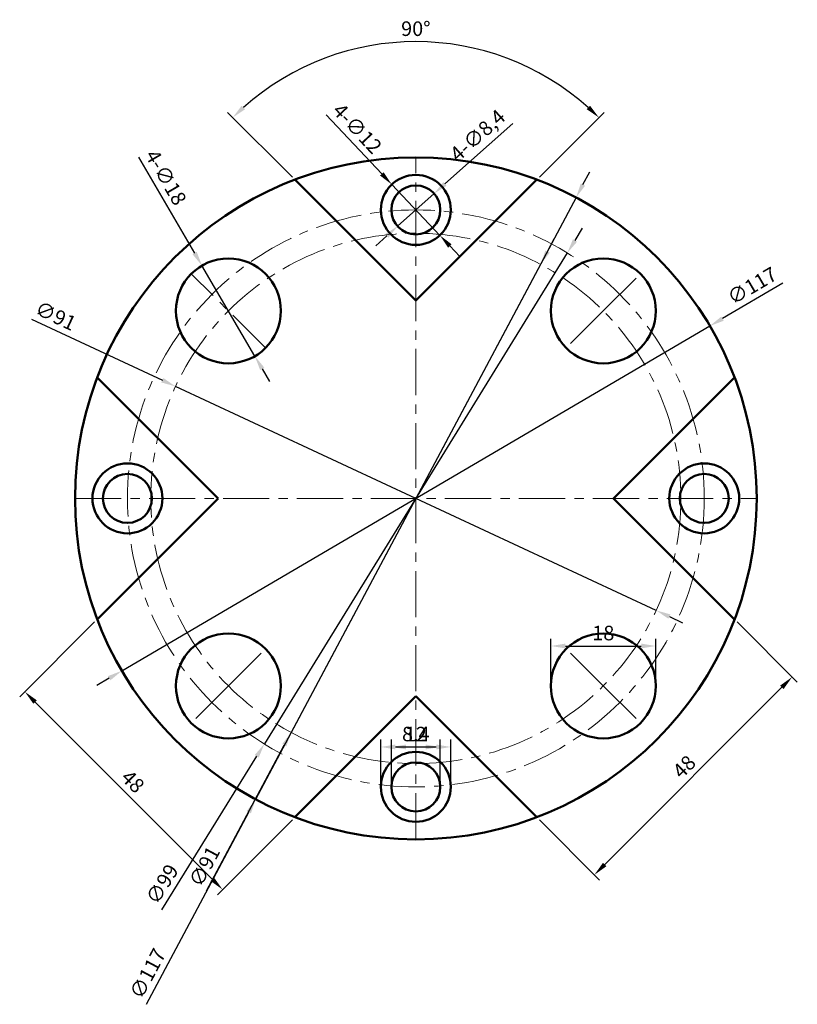
# Model space of a CAD drawing. Units: millimetres. Extents: x 3034 to 3167, y 1610 to 1779.
import ezdxf

# ---------------------------------------------------------------- set-up
doc = ezdxf.new("R2010")
doc.units = ezdxf.units.MM
doc.linetypes.add('CENTER', pattern=[50.8, 31.75, -6.35, 6.35, -6.35])
for name, color, linetype, lineweight in [('M-CNTR', 4, 'CENTER', 18), ('M-DIMS', 2, 'Continuous', 25), ('M-OUTL', 7, 'Continuous', 50)]:
    doc.layers.add(name, color=color, linetype=linetype, lineweight=lineweight)
doc.styles.get("Standard").update_dxf_attribs({"font": 'arial.ttf'})
doc.dimstyles.new('ISO-25', dxfattribs={"dimtxt": 2.5, "dimasz": 2.5, "dimexe": 1.25, "dimexo": 0.625, "dimtad": 1, "dimtxsty": 'Standard', "dimcen": 2.5, "dimadec": 0, "dimazin": 0, "dimtfac": 1, "dimtmove": 0, "dimatfit": 3, "dimfxl": 1, "dimarcsym": 0})

# ---------------------------------------------------------------- blocks, each defined once
blk = doc.blocks.new('*U1')
for radius in [6, 4.2]:
    blk.add_circle((0, 0), radius)
blk = doc.blocks.new('*U2')
at = {"layer": 'M-OUTL', "color": 0, "linetype": 'ByBlock', "lineweight": -2, "transparency": 16777216}
blk.add_blockref('*U1', (3101.53, 1745.97), dxfattribs=at)
for p, rotation in [((3052.03, 1696.47), 90), ((3151.03, 1696.47), 270.0000000000001), ((3101.53, 1646.97), 180)]:
    blk.add_blockref('*U1', p, dxfattribs=dict(at, rotation=rotation))
blk = doc.blocks.new('*U3')
blk.add_circle((0, 0), 9)
blk = doc.blocks.new('*U4')
at = {"layer": 'M-OUTL', "color": 0, "linetype": 'ByBlock', "lineweight": -2, "transparency": 16777216}
blk.add_blockref('*U3', (3069.36, 1728.64), dxfattribs=at)
for p, rotation in [((3133.71, 1728.64), 270), ((3069.36, 1664.29), 90.00000000000003), ((3133.71, 1664.29), 180)]:
    blk.add_blockref('*U3', p, dxfattribs=dict(at, rotation=rotation))
blk = doc.blocks.new('*D5')
at = {"layer": 'Defpoints', "color": 0, "transparency": 16777216}
for p in [(3064.82, 1736.41), (3073.9, 1720.87)]:
    blk.add_point(p, dxfattribs=at)
at = {"layer": 'M-DIMS', "color": 0, "lineweight": -2, "transparency": 16777216}
for p, q in [((3053.95, 1755.03), (3063.56, 1738.57)), ((3073.9, 1720.87), (3064.82, 1736.41)), ((3075.16, 1718.71), (3076.42, 1716.55))]:
    blk.add_line(p, q, dxfattribs=at)
at = {"layer": 'M-DIMS', "color": 0, "transparency": 16777216}
for points in [[(3063.92, 1738.78), (3063.2, 1738.36), (3064.82, 1736.41)], [(3075.52, 1718.92), (3074.8, 1718.5), (3073.9, 1720.87)]]:
    blk.add_solid(points, dxfattribs=at)
at = {"layer": 'M-DIMS', "color": 0, "transparency": 16777216, "insert": (3058.36, 1751.38), "char_height": 2.5, "attachment_point": 5, "rotation": 300.2839}
blk.add_mtext('4-∅18', dxfattribs=at)
blk = doc.blocks.new('*D6')
at = {"layer": 'Defpoints', "color": 0, "transparency": 16777216}
for p in [(3097.41, 1750.33), (3105.65, 1741.6)]:
    blk.add_point(p, dxfattribs=at)
at = {"layer": 'M-DIMS', "color": 0, "lineweight": -2, "transparency": 16777216}
for p, q in [((3086.14, 1762.27), (3095.7, 1752.15)), ((3105.65, 1741.6), (3097.41, 1750.33)), ((3107.37, 1739.78), (3109.08, 1737.97))]:
    blk.add_line(p, q, dxfattribs=at)
at = {"layer": 'M-DIMS', "color": 0, "transparency": 16777216}
for points in [[(3096, 1752.43), (3095.39, 1751.86), (3097.41, 1750.33)], [(3107.67, 1740.07), (3107.07, 1739.5), (3105.65, 1741.6)]]:
    blk.add_solid(points, dxfattribs=at)
at = {"layer": 'M-DIMS', "color": 0, "transparency": 16777216, "insert": (3091.26, 1759.72), "char_height": 2.5, "attachment_point": 5, "rotation": 313.3562}
blk.add_mtext('4-∅12', dxfattribs=at)
blk = doc.blocks.new('*D7')
at = {"layer": 'Defpoints', "color": 0, "transparency": 16777216}
for p in [(3104.66, 1748.76), (3098.4, 1743.17)]:
    blk.add_point(p, dxfattribs=at)
at = {"layer": 'M-DIMS', "color": 0, "lineweight": -2, "transparency": 16777216}
for p, q in [((3118.15, 1760.82), (3106.53, 1750.43)), ((3098.4, 1743.17), (3104.66, 1748.76)), ((3096.54, 1741.5), (3094.67, 1739.83))]:
    blk.add_line(p, q, dxfattribs=at)
at = {"layer": 'M-DIMS', "color": 0, "transparency": 16777216}
for points in [[(3106.25, 1750.74), (3106.81, 1750.12), (3104.66, 1748.76)], [(3096.26, 1741.81), (3096.82, 1741.19), (3098.4, 1743.17)]]:
    blk.add_solid(points, dxfattribs=at)
at = {"layer": 'M-DIMS', "color": 0, "transparency": 16777216, "insert": (3112.34, 1758.53), "char_height": 2.5, "attachment_point": 5, "rotation": 41.7886}
blk.add_mtext('4-∅8,4', dxfattribs=at)
blk = doc.blocks.new('*D8')
at = {"layer": 'Defpoints', "color": 0, "transparency": 16777216}
for p in [(3152, 1726.05), (3051.06, 1666.88)]:
    blk.add_point(p, dxfattribs=at)
at = {"layer": 'M-DIMS', "color": 0, "lineweight": -2, "transparency": 16777216}
for p, q in [((3164.51, 1733.38), (3154.16, 1727.31)), ((3051.06, 1666.88), (3152, 1726.05)), ((3048.91, 1665.62), (3046.75, 1664.35))]:
    blk.add_line(p, q, dxfattribs=at)
at = {"layer": 'M-DIMS', "color": 0, "transparency": 16777216}
for points in [[(3153.95, 1727.67), (3154.37, 1726.95), (3152, 1726.05)], [(3048.7, 1665.98), (3049.12, 1665.26), (3051.06, 1666.88)]]:
    blk.add_solid(points, dxfattribs=at)
at = {"layer": 'M-DIMS', "color": 0, "transparency": 16777216, "insert": (3159.41, 1732.68), "char_height": 2.5, "attachment_point": 5, "rotation": 30.3783}
blk.add_mtext('∅117', dxfattribs=at)
blk = doc.blocks.new('*D9')
at = {"layer": 'Defpoints', "color": 0, "transparency": 16777216}
for p in [(3060.29, 1715.68), (3142.78, 1677.25)]:
    blk.add_point(p, dxfattribs=at)
at = {"layer": 'M-DIMS', "color": 0, "lineweight": -2, "transparency": 16777216}
for p, q in [((3035.54, 1727.21), (3058.02, 1716.74)), ((3142.78, 1677.25), (3060.29, 1715.68)), ((3145.04, 1676.19), (3147.31, 1675.14))]:
    blk.add_line(p, q, dxfattribs=at)
at = {"layer": 'M-DIMS', "color": 0, "transparency": 16777216}
for points in [[(3058.2, 1717.12), (3057.85, 1716.36), (3060.29, 1715.68)], [(3145.22, 1676.57), (3144.87, 1675.82), (3142.78, 1677.25)]]:
    blk.add_solid(points, dxfattribs=at)
at = {"layer": 'M-DIMS', "color": 0, "transparency": 16777216, "insert": (3039.58, 1727.51), "char_height": 2.5, "attachment_point": 5, "rotation": 335.0174}
blk.add_mtext('∅91', dxfattribs=at)
blk = doc.blocks.new('*D10')
at = {"layer": 'Defpoints', "color": 0, "transparency": 16777216}
for p in [(3156.23, 1675.71), (3122.29, 1641.77), (3132.18, 1631.88)]:
    blk.add_point(p, dxfattribs=at)
at = {"layer": 'M-DIMS', "color": 0, "lineweight": -2, "transparency": 16777216}
for p, q in [((3156.67, 1675.27), (3167, 1664.93)), ((3164.35, 1664.05), (3133.95, 1633.65)), ((3122.73, 1641.33), (3133.06, 1630.99))]:
    blk.add_line(p, q, dxfattribs=at)
at = {"layer": 'M-DIMS', "color": 0, "transparency": 16777216}
for points in [[(3164.06, 1664.35), (3164.65, 1663.76), (3166.12, 1665.82)], [(3133.65, 1633.94), (3134.24, 1633.35), (3132.18, 1631.88)]]:
    blk.add_solid(points, dxfattribs=at)
at = {"layer": 'M-DIMS', "color": 0, "transparency": 16777216, "insert": (3147.81, 1650.19), "char_height": 2.5, "attachment_point": 5, "rotation": 45}
blk.add_mtext('48', dxfattribs=at)
blk = doc.blocks.new('*D11')
at = {"layer": 'Defpoints', "color": 0, "transparency": 16777216}
for p in [(3046.84, 1675.71), (3034.42, 1663.29), (3080.78, 1641.77)]:
    blk.add_point(p, dxfattribs=at)
at = {"layer": 'M-DIMS', "color": 0, "lineweight": -2, "transparency": 16777216}
for p, q in [((3046.4, 1675.27), (3033.54, 1662.41)), ((3066.59, 1631.12), (3036.19, 1661.53)), ((3080.34, 1641.33), (3067.48, 1628.47))]:
    blk.add_line(p, q, dxfattribs=at)
at = {"layer": 'M-DIMS', "color": 0, "transparency": 16777216}
for points in [[(3036.48, 1661.82), (3035.89, 1661.23), (3034.42, 1663.29)], [(3066.89, 1631.42), (3066.3, 1630.83), (3068.36, 1629.35)]]:
    blk.add_solid(points, dxfattribs=at)
at = {"layer": 'M-DIMS', "color": 0, "transparency": 16777216, "insert": (3052.74, 1647.67), "char_height": 2.5, "attachment_point": 5, "rotation": 315}
blk.add_mtext('48', dxfattribs=at)
blk = doc.blocks.new('*D12')
at = {"layer": 'Defpoints', "color": 0, "transparency": 16777216}
for p in [(3113.03, 1773.33), (3080.78, 1751.16), (3122.29, 1751.16), (3116.74, 1745.61), (3101.53, 1730.41)]:
    blk.add_point(p, dxfattribs=at)
at = {"layer": 'M-DIMS', "color": 0, "lineweight": -2, "transparency": 16777216}
for p, q in [((3080.34, 1751.6), (3069.23, 1762.71)), ((3122.73, 1751.6), (3133.84, 1762.71))]:
    blk.add_line(p, q, dxfattribs=at)
blk.add_arc((3101.53, 1730.41), 44.43, 48.2241, 131.7759, dxfattribs=at)
at = {"layer": 'M-DIMS', "color": 0, "transparency": 16777216}
for points in [[(3072.22, 1763.24), (3071.64, 1763.85), (3070.11, 1761.83)], [(3131.42, 1763.85), (3130.85, 1763.24), (3132.95, 1761.83)]]:
    blk.add_solid(points, dxfattribs=at)
at = {"layer": 'M-DIMS', "color": 0, "transparency": 16777216, "insert": (3101.53, 1776.74), "char_height": 2.5, "attachment_point": 5}
blk.add_mtext('90°', dxfattribs=at)
blk = doc.blocks.new('*D13')
at = {"layer": 'Defpoints', "color": 0, "transparency": 16777216}
for p in [(3142.71, 1671.14), (3124.71, 1664.29), (3142.71, 1664.29)]:
    blk.add_point(p, dxfattribs=at)
at = {"layer": 'M-DIMS', "color": 0, "lineweight": -2, "transparency": 16777216}
for p, q in [((3124.71, 1664.92), (3124.71, 1672.39)), ((3127.21, 1671.14), (3140.21, 1671.14)), ((3142.71, 1664.92), (3142.71, 1672.39))]:
    blk.add_line(p, q, dxfattribs=at)
at = {"layer": 'M-DIMS', "color": 0, "transparency": 16777216}
for points in [[(3127.21, 1671.56), (3127.21, 1670.73), (3124.71, 1671.14)], [(3140.21, 1671.56), (3140.21, 1670.73), (3142.71, 1671.14)]]:
    blk.add_solid(points, dxfattribs=at)
at = {"layer": 'M-DIMS', "color": 0, "transparency": 16777216, "insert": (3133.71, 1673.04), "char_height": 2.5, "attachment_point": 5}
blk.add_mtext('18', dxfattribs=at)
blk = doc.blocks.new('*D14')
at = {"layer": 'Defpoints', "color": 0, "transparency": 16777216}
for p in [(3105.73, 1653.82), (3097.33, 1646.97), (3105.73, 1646.97)]:
    blk.add_point(p, dxfattribs=at)
at = {"layer": 'M-DIMS', "color": 0, "lineweight": -2, "transparency": 16777216}
for p, q in [((3097.33, 1647.59), (3097.33, 1655.07)), ((3105.73, 1647.59), (3105.73, 1655.07)), ((3099.83, 1653.82), (3103.23, 1653.82))]:
    blk.add_line(p, q, dxfattribs=at)
at = {"layer": 'M-DIMS', "color": 0, "transparency": 16777216}
for points in [[(3099.83, 1654.23), (3099.83, 1653.4), (3097.33, 1653.82)], [(3103.23, 1654.23), (3103.23, 1653.4), (3105.73, 1653.82)]]:
    blk.add_solid(points, dxfattribs=at)
at = {"layer": 'M-DIMS', "color": 0, "transparency": 16777216, "insert": (3101.53, 1655.72), "char_height": 2.5, "attachment_point": 5}
blk.add_mtext('8.4', dxfattribs=at)
blk = doc.blocks.new('*D15')
at = {"layer": 'Defpoints', "color": 0, "transparency": 16777216}
for p in [(3107.53, 1653.82), (3095.53, 1646.97), (3107.53, 1646.97)]:
    blk.add_point(p, dxfattribs=at)
at = {"layer": 'M-DIMS', "color": 0, "lineweight": -2, "transparency": 16777216}
for p, q in [((3095.53, 1647.59), (3095.53, 1655.07)), ((3107.53, 1647.59), (3107.53, 1655.07)), ((3098.03, 1653.82), (3105.03, 1653.82))]:
    blk.add_line(p, q, dxfattribs=at)
at = {"layer": 'M-DIMS', "color": 0, "transparency": 16777216}
for points in [[(3098.03, 1654.23), (3098.03, 1653.4), (3095.53, 1653.82)], [(3105.03, 1654.23), (3105.03, 1653.4), (3107.53, 1653.82)]]:
    blk.add_solid(points, dxfattribs=at)
at = {"layer": 'M-DIMS', "color": 0, "transparency": 16777216, "insert": (3101.53, 1655.7), "char_height": 2.5, "attachment_point": 5}
blk.add_mtext('12', dxfattribs=at)
blk = doc.blocks.new('*D16')
at = {"layer": 'Defpoints', "color": 0, "transparency": 16777216}
for p in [(3129.03, 1748.1), (3074.03, 1644.83)]:
    blk.add_point(p, dxfattribs=at)
at = {"layer": 'M-DIMS', "color": 0, "lineweight": -2, "transparency": 16777216}
for p, q in [((3130.21, 1750.31), (3131.38, 1752.51)), ((3129.03, 1748.1), (3074.03, 1644.83)), ((3055.3, 1609.66), (3072.86, 1642.62))]:
    blk.add_line(p, q, dxfattribs=at)
at = {"layer": 'M-DIMS', "color": 0, "transparency": 16777216}
for points in [[(3129.84, 1750.5), (3130.58, 1750.11), (3129.03, 1748.1)], [(3072.49, 1642.82), (3073.23, 1642.43), (3074.03, 1644.83)]]:
    blk.add_solid(points, dxfattribs=at)
at = {"layer": 'M-DIMS', "color": 0, "transparency": 16777216, "insert": (3055.79, 1614.78), "char_height": 2.5, "attachment_point": 5, "rotation": 61.961}
blk.add_mtext('∅117', dxfattribs=at)
blk = doc.blocks.new('*D17')
at = {"layer": 'Defpoints', "color": 0, "transparency": 16777216}
for p in [(3127.53, 1738.59), (3075.53, 1654.34)]:
    blk.add_point(p, dxfattribs=at)
at = {"layer": 'M-DIMS', "color": 0, "lineweight": -2, "transparency": 16777216}
for p, q in [((3128.85, 1740.71), (3130.16, 1742.84)), ((3127.53, 1738.59), (3075.53, 1654.34)), ((3057.95, 1625.86), (3074.22, 1652.22))]:
    blk.add_line(p, q, dxfattribs=at)
at = {"layer": 'M-DIMS', "color": 0, "transparency": 16777216}
for points in [[(3128.49, 1740.93), (3129.2, 1740.5), (3127.53, 1738.59)], [(3073.87, 1652.43), (3074.57, 1652), (3075.53, 1654.34)]]:
    blk.add_solid(points, dxfattribs=at)
at = {"layer": 'M-DIMS', "color": 0, "transparency": 16777216, "insert": (3058.26, 1630.11), "char_height": 2.5, "attachment_point": 5, "rotation": 58.315}
blk.add_mtext('∅99', dxfattribs=at)
blk = doc.blocks.new('*D18')
at = {"layer": 'Defpoints', "color": 0, "transparency": 16777216}
for p in [(3122.95, 1736.61), (3080.12, 1656.32)]:
    blk.add_point(p, dxfattribs=at)
at = {"layer": 'M-DIMS', "color": 0, "lineweight": -2, "transparency": 16777216}
for p, q in [((3124.12, 1738.82), (3125.3, 1741.02)), ((3122.95, 1736.61), (3080.12, 1656.32)), ((3065.61, 1629.11), (3078.94, 1654.11))]:
    blk.add_line(p, q, dxfattribs=at)
at = {"layer": 'M-DIMS', "color": 0, "transparency": 16777216}
for points in [[(3123.75, 1739.01), (3124.49, 1738.62), (3122.95, 1736.61)], [(3078.58, 1654.31), (3079.31, 1653.92), (3080.12, 1656.32)]]:
    blk.add_solid(points, dxfattribs=at)
at = {"layer": 'M-DIMS', "color": 0, "transparency": 16777216, "insert": (3065.53, 1633.16), "char_height": 2.5, "attachment_point": 5, "rotation": 61.9261}
blk.add_mtext('∅91', dxfattribs=at)

msp = doc.modelspace()

# ---------------------------------------------------------------- linework, layer by layer
at = {"layer": 'M-CNTR', "ltscale": 0.25, "transparency": 33554534}
for p, q in [((3101.533, 1637.965), (3101.533, 1754.965)), ((3075.724, 1722.275), (3062.996, 1735.003)), ((3133.706, 1728.639), (3140.07, 1735.003)), ((3133.706, 1728.639), (3127.342, 1722.275)), ((3043.033, 1696.465), (3160.033, 1696.465)), ((3069.36, 1664.292), (3075.724, 1670.656)), ((3133.706, 1664.292), (3127.342, 1670.656)), ((3069.36, 1664.292), (3062.996, 1657.928)), ((3133.706, 1664.292), (3140.07, 1657.928))]:
    msp.add_line(p, q, dxfattribs=at)
for radius in [49.5, 45.5]:
    msp.add_circle((3101.533, 1696.465), radius, dxfattribs=at)
at = {"layer": 'M-OUTL'}
for p, q in [((3101.533, 1730.406), (3080.779, 1751.16)), ((3116.736, 1745.609), (3122.287, 1751.16)), ((3116.736, 1745.609), (3101.533, 1730.406)), ((3067.592, 1696.465), (3046.838, 1717.219)), ((3150.677, 1711.668), (3156.228, 1717.219)), ((3150.677, 1711.668), (3139.558, 1700.549)), ((3139.558, 1700.549), (3135.474, 1696.465)), ((3052.389, 1681.262), (3067.592, 1696.465)), ((3150.677, 1681.262), (3135.474, 1696.465)), ((3052.389, 1681.262), (3046.838, 1675.712)), ((3150.677, 1681.262), (3156.228, 1675.712)), ((3086.33, 1647.321), (3101.533, 1662.524)), ((3116.736, 1647.321), (3101.533, 1662.524)), ((3086.33, 1647.321), (3080.779, 1641.77)), ((3116.736, 1647.321), (3122.287, 1641.77))]:
    msp.add_line(p, q, dxfattribs=at)
msp.add_circle((3101.533, 1696.465), 58.5, dxfattribs=at)

# ---------------------------------------------------------------- block references
for name in ['*U2', '*U4']:
    msp.add_blockref(name, (0, 0), dxfattribs=at)

# ---------------------------------------------------------------- dimensions: what is measured, and where the dimension line sits
at = {"layer": 'M-DIMS'}
dim = msp.add_angular_dim_2l(base=(3113.033, 1773.326), line1=((3116.736, 1745.609), (3122.287, 1751.16)), line2=((3101.533, 1730.406), (3080.779, 1751.16)), dimstyle='ISO-25', override={"dimclrd": 0, "dimclre": 0, "dimclrt": 0}, dxfattribs=at)
dim.commit()
dim.dimension.update_dxf_attribs({"geometry": '*D12', "text_midpoint": (3101.533, 1776.742)})
for p1, p2, picture, middle in [((3105.652, 1741.603), (3097.414, 1750.328), '*D6', (3089.822, 1758.368)), ((3098.402, 1743.166), (3104.665, 1748.764), '*D7', (3113.787, 1756.917)), ((3073.898, 1720.867), (3064.821, 1736.41), '*D5', (3056.659, 1750.388))]:
    dim = msp.add_diameter_dim_2p(p1=p1, p2=p2, text='4-<>', dimstyle='ISO-25', override={"dimclrd": 0, "dimclre": 0, "dimclrt": 0}, dxfattribs=at)
    dim.commit()
    dim.dimension.update_dxf_attribs({"geometry": picture, "text_midpoint": middle, "dimtype": 163})
for p1, p2, override, picture, middle in [((3129.032, 1748.099), (3074.034, 1644.832), {"dimdec": 0, "dimlfac": 1, "dimrnd": 0, "dimzin": 0, "dimdsep": 46, "dimlunit": 2}, '*D16', (3057.534, 1613.851)), ((3127.533, 1738.587), (3075.533, 1654.343), {"dimdec": 0, "dimlfac": 1, "dimrnd": 0, "dimzin": 0, "dimdsep": 46, "dimlunit": 2}, '*D17', (3059.933, 1629.07)), ((3122.946, 1736.612), (3080.12, 1656.319), {"dimdec": 0, "dimlfac": 1, "dimrnd": 0, "dimzin": 0, "dimdsep": 46, "dimlunit": 2}, '*D18', (3067.273, 1632.231)), ((3142.776, 1677.249), (3060.29, 1715.682), {"dimclrd": 0, "dimclre": 0, "dimclrt": 0}, '*D9', (3038.746, 1725.72))]:
    dim = msp.add_diameter_dim_2p(p1=p1, p2=p2, dimstyle='ISO-25', override=override, dxfattribs=at)
    dim.commit()
    dim.dimension.update_dxf_attribs({"geometry": picture, "text_midpoint": middle, "dimtype": 163})
dim = msp.add_diameter_dim_2p(p1=(3051.065, 1666.881), p2=(3152.001, 1726.049), dimstyle='ISO-25', override={"dimclrd": 0, "dimclre": 0, "dimclrt": 0}, dxfattribs=at)
dim.commit()
dim.dimension.update_dxf_attribs({"geometry": '*D8', "text_midpoint": (3159.413, 1732.679)})
for p1, p2, distance, picture, middle in [((3080.779, 1641.77), (3046.838, 1675.712), 17.561, '*D11', (3052.736, 1647.668)), ((3156.228, 1675.712), (3122.287, 1641.77), 13.99, '*D10', (3147.806, 1650.193))]:
    dim = msp.add_aligned_dim(p1=p1, p2=p2, distance=distance, dimstyle='ISO-25', override={"dimclrd": 0, "dimclre": 0, "dimclrt": 0}, dxfattribs=at)
    dim.commit()
    dim.dimension.update_dxf_attribs({"geometry": picture, "text_midpoint": middle})
for base, p1, p2, override, picture, middle in [((3142.706, 1671.142), (3124.706, 1664.292), (3142.706, 1664.292), {"dimdec": 0, "dimlfac": 1, "dimrnd": 0, "dimzin": 0, "dimdsep": 46, "dimlunit": 2}, '*D13', (3133.706, 1673.043)), ((3105.733, 1653.815), (3097.333, 1646.965), (3105.733, 1646.965), {"dimdec": 1, "dimlfac": 1, "dimrnd": 0, "dimzin": 0, "dimdsep": 46, "dimlunit": 2}, '*D14', (3101.533, 1655.717)), ((3107.533, 1653.815), (3095.533, 1646.965), (3107.533, 1646.965), {"dimdec": 0, "dimlfac": 1, "dimrnd": 0, "dimzin": 0, "dimdsep": 46, "dimlunit": 2}, '*D15', (3101.533, 1655.695))]:
    dim = msp.add_linear_dim(base=base, p1=p1, p2=p2, dimstyle='ISO-25', override=override, dxfattribs=at)
    dim.commit()
    dim.dimension.update_dxf_attribs({"geometry": picture, "text_midpoint": middle})

doc.saveas('drawing.dxf')
